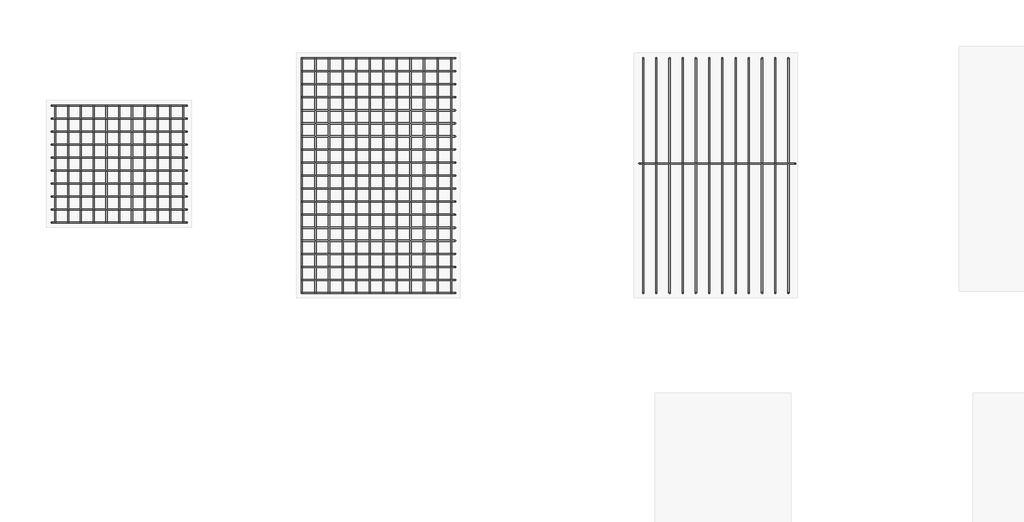
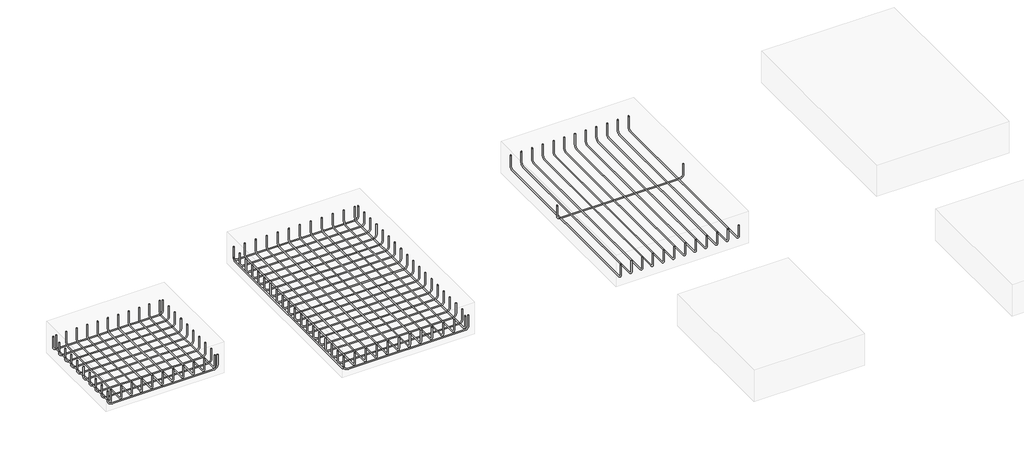
# One storey, part 2 of 2: 6 reinforcing bars.
"""IFC4 building model written with IfcOpenShell, lengths in millimetres."""

from ifc_helpers import new_model, si_unit, point, frame, origin, place, context, project, spatial, polyline, circle_curve, trimmed, segment, composite_curve, source, transform, mapped, element, save
from ifc_brep_helpers import swept_disk

model = new_model("IFC4")

# Units and contexts
model_context = context("Model", 3, world=origin())
ifc_project = project(units=[si_unit("LENGTHUNIT", "METRE", prefix="MILLI")], contexts=[model_context])

# Site, building, storey
site = spatial("IfcSite", under=ifc_project)
building = spatial("IfcBuilding", under=site)
storey = spatial("IfcBuildingStorey", under=building, Elevation=-2133.6)

# Reinforcing bars
placement = place(None, origin())
reinforcing_bar_shape = source(origin(), model_context, "Body", "SolidModel", [
    swept_disk(composite_curve([segment(polyline([(-14776.9377753, 5351.4047256, -2333.6), (-14776.9377753, 5351.4047256, -2480.9)]), True, "CONTINUOUS"), segment(trimmed(circle_curve(frame((-14823.2877753, 5351.4047256, -2480.9), z_axis=(0.0, 1.0, 0.0), x_axis=(46.349999999998545, 0.0, 0.0)), 46.35), [point((-14776.9377753, 5351.4047256, -2480.9))], [point((-14823.2877753, 5351.4047256, -2527.25))], True, "CARTESIAN"), True, "CONTINUOUS"), segment(polyline([(-14823.2877753, 5351.4047256, -2527.25), (-16217.8877753, 5351.4047256, -2527.25)]), True, "CONTINUOUS"), segment(trimmed(circle_curve(frame((-16217.8877753, 5351.4047256, -2480.9), z_axis=(0.0, 1.0, 0.0), x_axis=(0.0, 0.0, -46.34999999999991)), 46.35), [point((-16217.8877753, 5351.4047256, -2527.25))], [point((-16264.2377753, 5351.4047256, -2480.9))], True, "CARTESIAN"), True, "CONTINUOUS"), segment(polyline([(-16264.2377753, 5351.4047256, -2480.9), (-16264.2377753, 5351.4047256, -2333.6)]), True, "CONTINUOUS")], self_intersect=False), 6.35),
])
element("IfcReinforcingBar", 1, at=placement, inside=storey, context=model_context, shape_type="MappedRepresentation", body=[
    mapped(reinforcing_bar_shape, transform((0.0, 0.0, 0.0), x_axis=(1.0, 0.0, 0.0), y_axis=(0.0, 1.0, 0.0), z_axis=(0.0, 0.0, 1.0))),
    mapped(reinforcing_bar_shape, transform((0.0, -143.0333333, 0.0), x_axis=(1.0, 0.0, 0.0), y_axis=(0.0, 1.0, 0.0), z_axis=(0.0, 0.0, 1.0))),
    mapped(reinforcing_bar_shape, transform((0.0, -286.0666667, 0.0), x_axis=(1.0, 0.0, 0.0), y_axis=(0.0, 1.0, 0.0), z_axis=(0.0, 0.0, 1.0))),
    mapped(reinforcing_bar_shape, transform((0.0, -429.1, 0.0), x_axis=(1.0, 0.0, 0.0), y_axis=(0.0, 1.0, 0.0), z_axis=(0.0, 0.0, 1.0))),
    mapped(reinforcing_bar_shape, transform((0.0, -572.1333333, 0.0), x_axis=(1.0, 0.0, 0.0), y_axis=(0.0, 1.0, 0.0), z_axis=(0.0, 0.0, 1.0))),
    mapped(reinforcing_bar_shape, transform((0.0, -715.1666667, 0.0), x_axis=(1.0, 0.0, 0.0), y_axis=(0.0, 1.0, 0.0), z_axis=(0.0, 0.0, 1.0))),
    mapped(reinforcing_bar_shape, transform((0.0, -858.2, 0.0), x_axis=(1.0, 0.0, 0.0), y_axis=(0.0, 1.0, 0.0), z_axis=(0.0, 0.0, 1.0))),
    mapped(reinforcing_bar_shape, transform((0.0, -1001.2333333, 0.0), x_axis=(1.0, 0.0, 0.0), y_axis=(0.0, 1.0, 0.0), z_axis=(0.0, 0.0, 1.0))),
    mapped(reinforcing_bar_shape, transform((0.0, -1144.2666667, 0.0), x_axis=(1.0, 0.0, 0.0), y_axis=(0.0, 1.0, 0.0), z_axis=(0.0, 0.0, 1.0))),
    mapped(reinforcing_bar_shape, transform((0.0, -1287.3, 0.0), x_axis=(1.0, 0.0, 0.0), y_axis=(0.0, 1.0, 0.0), z_axis=(0.0, 0.0, 1.0))),
])
reinforcing_bar_2_shape = source(origin(), model_context, "Body", "SolidModel", [
    swept_disk(composite_curve([segment(polyline([(-16224.2377753, 5351.4047256, -2327.3038613), (-16224.2377753, 5351.4047256, -2474.6038613)]), True, "CONTINUOUS"), segment(trimmed(circle_curve(frame((-16224.2377753, 5305.0547256, -2474.6038613), z_axis=(-1.0, 0.0, 0.0), x_axis=(0.0, 46.350000000000364, 0.0)), 46.35), [point((-16224.2377753, 5351.4047256, -2474.6038613))], [point((-16224.2377753, 5305.0547256, -2520.9538613))], True, "CARTESIAN"), True, "CONTINUOUS"), segment(polyline([(-16224.2377753, 5305.0547256, -2520.9538613), (-16224.2377753, 4110.4547256, -2520.9538613)]), True, "CONTINUOUS"), segment(trimmed(circle_curve(frame((-16224.2377753, 4110.4547256, -2474.6038613), z_axis=(-1.0, 0.0, 0.0), x_axis=(0.0, 0.0, -46.34999999999991)), 46.35), [point((-16224.2377753, 4110.4547256, -2520.9538613))], [point((-16224.2377753, 4064.1047256, -2474.6038613))], True, "CARTESIAN"), True, "CONTINUOUS"), segment(polyline([(-16224.2377753, 4064.1047256, -2474.6038613), (-16224.2377753, 4064.1047256, -2327.3038613)]), True, "CONTINUOUS")], self_intersect=False), 6.35),
])
element("IfcReinforcingBar", 2, at=placement, inside=storey, context=model_context, shape_type="MappedRepresentation", body=[
    mapped(reinforcing_bar_2_shape, transform((0.0, 0.0, 0.0), x_axis=(1.0, 0.0, 0.0), y_axis=(0.0, 1.0, 0.0), z_axis=(0.0, 0.0, 1.0))),
    mapped(reinforcing_bar_2_shape, transform((140.73, 0.0, 0.0), x_axis=(1.0, 0.0, 0.0), y_axis=(0.0, 1.0, 0.0), z_axis=(0.0, 0.0, 1.0))),
    mapped(reinforcing_bar_2_shape, transform((281.46, 0.0, 0.0), x_axis=(1.0, 0.0, 0.0), y_axis=(0.0, 1.0, 0.0), z_axis=(0.0, 0.0, 1.0))),
    mapped(reinforcing_bar_2_shape, transform((422.19, 0.0, 0.0), x_axis=(1.0, 0.0, 0.0), y_axis=(0.0, 1.0, 0.0), z_axis=(0.0, 0.0, 1.0))),
    mapped(reinforcing_bar_2_shape, transform((562.92, 0.0, 0.0), x_axis=(1.0, 0.0, 0.0), y_axis=(0.0, 1.0, 0.0), z_axis=(0.0, 0.0, 1.0))),
    mapped(reinforcing_bar_2_shape, transform((703.65, 0.0, 0.0), x_axis=(1.0, 0.0, 0.0), y_axis=(0.0, 1.0, 0.0), z_axis=(0.0, 0.0, 1.0))),
    mapped(reinforcing_bar_2_shape, transform((844.38, 0.0, 0.0), x_axis=(1.0, 0.0, 0.0), y_axis=(0.0, 1.0, 0.0), z_axis=(0.0, 0.0, 1.0))),
    mapped(reinforcing_bar_2_shape, transform((985.11, 0.0, 0.0), x_axis=(1.0, 0.0, 0.0), y_axis=(0.0, 1.0, 0.0), z_axis=(0.0, 0.0, 1.0))),
    mapped(reinforcing_bar_2_shape, transform((1125.84, 0.0, 0.0), x_axis=(1.0, 0.0, 0.0), y_axis=(0.0, 1.0, 0.0), z_axis=(0.0, 0.0, 1.0))),
    mapped(reinforcing_bar_2_shape, transform((1266.57, 0.0, 0.0), x_axis=(1.0, 0.0, 0.0), y_axis=(0.0, 1.0, 0.0), z_axis=(0.0, 0.0, 1.0))),
    mapped(reinforcing_bar_2_shape, transform((1407.3, 0.0, 0.0), x_axis=(1.0, 0.0, 0.0), y_axis=(0.0, 1.0, 0.0), z_axis=(0.0, 0.0, 1.0))),
])
reinforcing_bar_3_shape = source(origin(), model_context, "Body", "SolidModel", [
    swept_disk(composite_curve([segment(polyline([(-11823.152732, 5876.4047256, -2333.6), (-11823.152732, 5876.4047256, -2480.9)]), True, "CONTINUOUS"), segment(trimmed(circle_curve(frame((-11869.502732, 5876.4047256, -2480.9), z_axis=(0.0, 1.0, 0.0), x_axis=(46.350000000000364, 0.0, 0.0)), 46.35), [point((-11823.152732, 5876.4047256, -2480.9))], [point((-11869.502732, 5876.4047256, -2527.25))], True, "CARTESIAN"), True, "CONTINUOUS"), segment(polyline([(-11869.502732, 5876.4047256, -2527.25), (-13464.102732, 5876.4047256, -2527.25)]), True, "CONTINUOUS"), segment(trimmed(circle_curve(frame((-13464.102732, 5876.4047256, -2480.9), z_axis=(0.0, 1.0, 0.0), x_axis=(0.0, 0.0, -46.34999999999991)), 46.35), [point((-13464.102732, 5876.4047256, -2527.25))], [point((-13510.452732, 5876.4047256, -2480.9))], True, "CARTESIAN"), True, "CONTINUOUS"), segment(polyline([(-13510.452732, 5876.4047256, -2480.9), (-13510.452732, 5876.4047256, -2333.6)]), True, "CONTINUOUS")], self_intersect=False), 6.35),
])
element("IfcReinforcingBar", 3, at=placement, inside=storey, context=model_context, shape_type="MappedRepresentation", body=[
    mapped(reinforcing_bar_3_shape, transform((0.0, 0.0, 0.0), x_axis=(1.0, 0.0, 0.0), y_axis=(0.0, 1.0, 0.0), z_axis=(0.0, 0.0, 1.0))),
    mapped(reinforcing_bar_3_shape, transform((0.0, -143.7388889, 0.0), x_axis=(1.0, 0.0, 0.0), y_axis=(0.0, 1.0, 0.0), z_axis=(0.0, 0.0, 1.0))),
    mapped(reinforcing_bar_3_shape, transform((0.0, -287.4777778, 0.0), x_axis=(1.0, 0.0, 0.0), y_axis=(0.0, 1.0, 0.0), z_axis=(0.0, 0.0, 1.0))),
    mapped(reinforcing_bar_3_shape, transform((0.0, -431.2166667, 0.0), x_axis=(1.0, 0.0, 0.0), y_axis=(0.0, 1.0, 0.0), z_axis=(0.0, 0.0, 1.0))),
    mapped(reinforcing_bar_3_shape, transform((0.0, -574.9555556, 0.0), x_axis=(1.0, 0.0, 0.0), y_axis=(0.0, 1.0, 0.0), z_axis=(0.0, 0.0, 1.0))),
    mapped(reinforcing_bar_3_shape, transform((0.0, -718.6944444, 0.0), x_axis=(1.0, 0.0, 0.0), y_axis=(0.0, 1.0, 0.0), z_axis=(0.0, 0.0, 1.0))),
    mapped(reinforcing_bar_3_shape, transform((0.0, -862.4333333, 0.0), x_axis=(1.0, 0.0, 0.0), y_axis=(0.0, 1.0, 0.0), z_axis=(0.0, 0.0, 1.0))),
    mapped(reinforcing_bar_3_shape, transform((0.0, -1006.1722222, 0.0), x_axis=(1.0, 0.0, 0.0), y_axis=(0.0, 1.0, 0.0), z_axis=(0.0, 0.0, 1.0))),
    mapped(reinforcing_bar_3_shape, transform((0.0, -1149.9111111, 0.0), x_axis=(1.0, 0.0, 0.0), y_axis=(0.0, 1.0, 0.0), z_axis=(0.0, 0.0, 1.0))),
    mapped(reinforcing_bar_3_shape, transform((0.0, -1293.65, 0.0), x_axis=(1.0, 0.0, 0.0), y_axis=(0.0, 1.0, 0.0), z_axis=(0.0, 0.0, 1.0))),
    mapped(reinforcing_bar_3_shape, transform((0.0, -1437.3888889, 0.0), x_axis=(1.0, 0.0, 0.0), y_axis=(0.0, 1.0, 0.0), z_axis=(0.0, 0.0, 1.0))),
    mapped(reinforcing_bar_3_shape, transform((0.0, -1581.1277778, 0.0), x_axis=(1.0, 0.0, 0.0), y_axis=(0.0, 1.0, 0.0), z_axis=(0.0, 0.0, 1.0))),
    mapped(reinforcing_bar_3_shape, transform((0.0, -1724.8666667, 0.0), x_axis=(1.0, 0.0, 0.0), y_axis=(0.0, 1.0, 0.0), z_axis=(0.0, 0.0, 1.0))),
    mapped(reinforcing_bar_3_shape, transform((0.0, -1868.6055556, 0.0), x_axis=(1.0, 0.0, 0.0), y_axis=(0.0, 1.0, 0.0), z_axis=(0.0, 0.0, 1.0))),
    mapped(reinforcing_bar_3_shape, transform((0.0, -2012.3444444, 0.0), x_axis=(1.0, 0.0, 0.0), y_axis=(0.0, 1.0, 0.0), z_axis=(0.0, 0.0, 1.0))),
    mapped(reinforcing_bar_3_shape, transform((0.0, -2156.0833333, 0.0), x_axis=(1.0, 0.0, 0.0), y_axis=(0.0, 1.0, 0.0), z_axis=(0.0, 0.0, 1.0))),
    mapped(reinforcing_bar_3_shape, transform((0.0, -2299.8222222, 0.0), x_axis=(1.0, 0.0, 0.0), y_axis=(0.0, 1.0, 0.0), z_axis=(0.0, 0.0, 1.0))),
    mapped(reinforcing_bar_3_shape, transform((0.0, -2443.5611111, 0.0), x_axis=(1.0, 0.0, 0.0), y_axis=(0.0, 1.0, 0.0), z_axis=(0.0, 0.0, 1.0))),
    mapped(reinforcing_bar_3_shape, transform((0.0, -2587.3, 0.0), x_axis=(1.0, 0.0, 0.0), y_axis=(0.0, 1.0, 0.0), z_axis=(0.0, 0.0, 1.0))),
])
reinforcing_bar_4_shape = source(origin(), model_context, "Body", "SolidModel", [
    swept_disk(composite_curve([segment(polyline([(-13510.452732, 5876.4047256, -2327.2198924), (-13510.452732, 5876.4047256, -2474.5198924)]), True, "CONTINUOUS"), segment(trimmed(circle_curve(frame((-13510.452732, 5830.0547256, -2474.5198924), z_axis=(-1.0, 0.0, 0.0), x_axis=(0.0, 46.350000000000364, 0.0)), 46.35), [point((-13510.452732, 5876.4047256, -2474.5198924))], [point((-13510.452732, 5830.0547256, -2520.8698924))], True, "CARTESIAN"), True, "CONTINUOUS"), segment(polyline([(-13510.452732, 5830.0547256, -2520.8698924), (-13510.452732, 3335.4547256, -2520.8698924)]), True, "CONTINUOUS"), segment(trimmed(circle_curve(frame((-13510.452732, 3335.4547256, -2474.5198924), z_axis=(-1.0, 0.0, 0.0), x_axis=(0.0, 0.0, -46.34999999999991)), 46.35), [point((-13510.452732, 3335.4547256, -2520.8698924))], [point((-13510.452732, 3289.1047256, -2474.5198924))], True, "CARTESIAN"), True, "CONTINUOUS"), segment(polyline([(-13510.452732, 3289.1047256, -2474.5198924), (-13510.452732, 3289.1047256, -2327.2198924)]), True, "CONTINUOUS")], self_intersect=False), 6.35),
])
element("IfcReinforcingBar", 4, at=placement, inside=storey, context=model_context, shape_type="MappedRepresentation", body=[
    mapped(reinforcing_bar_4_shape, transform((0.0, 0.0, 0.0), x_axis=(1.0, 0.0, 0.0), y_axis=(0.0, 1.0, 0.0), z_axis=(0.0, 0.0, 1.0))),
    mapped(reinforcing_bar_4_shape, transform((149.4666138, 0.0, 0.0), x_axis=(1.0, 0.0, 0.0), y_axis=(0.0, 1.0, 0.0), z_axis=(0.0, 0.0, 1.0))),
    mapped(reinforcing_bar_4_shape, transform((298.9332277, 0.0, 0.0), x_axis=(1.0, 0.0, 0.0), y_axis=(0.0, 1.0, 0.0), z_axis=(0.0, 0.0, 1.0))),
    mapped(reinforcing_bar_4_shape, transform((448.3998415, 0.0, 0.0), x_axis=(1.0, 0.0, 0.0), y_axis=(0.0, 1.0, 0.0), z_axis=(0.0, 0.0, 1.0))),
    mapped(reinforcing_bar_4_shape, transform((597.8664554, 0.0, 0.0), x_axis=(1.0, 0.0, 0.0), y_axis=(0.0, 1.0, 0.0), z_axis=(0.0, 0.0, 1.0))),
    mapped(reinforcing_bar_4_shape, transform((747.3330692, 0.0, 0.0), x_axis=(1.0, 0.0, 0.0), y_axis=(0.0, 1.0, 0.0), z_axis=(0.0, 0.0, 1.0))),
    mapped(reinforcing_bar_4_shape, transform((896.7996831, 0.0, 0.0), x_axis=(1.0, 0.0, 0.0), y_axis=(0.0, 1.0, 0.0), z_axis=(0.0, 0.0, 1.0))),
    mapped(reinforcing_bar_4_shape, transform((1046.2662969, 0.0, 0.0), x_axis=(1.0, 0.0, 0.0), y_axis=(0.0, 1.0, 0.0), z_axis=(0.0, 0.0, 1.0))),
    mapped(reinforcing_bar_4_shape, transform((1195.7329107, 0.0, 0.0), x_axis=(1.0, 0.0, 0.0), y_axis=(0.0, 1.0, 0.0), z_axis=(0.0, 0.0, 1.0))),
    mapped(reinforcing_bar_4_shape, transform((1345.1995246, 0.0, 0.0), x_axis=(1.0, 0.0, 0.0), y_axis=(0.0, 1.0, 0.0), z_axis=(0.0, 0.0, 1.0))),
    mapped(reinforcing_bar_4_shape, transform((1494.6661384, 0.0, 0.0), x_axis=(1.0, 0.0, 0.0), y_axis=(0.0, 1.0, 0.0), z_axis=(0.0, 0.0, 1.0))),
    mapped(reinforcing_bar_4_shape, transform((1644.1327523, 0.0, 0.0), x_axis=(1.0, 0.0, 0.0), y_axis=(0.0, 1.0, 0.0), z_axis=(0.0, 0.0, 1.0))),
])
element("IfcReinforcingBar", 5, at=placement, inside=storey, context=model_context, shape_type="SolidModel", body=[
    swept_disk(composite_curve([segment(polyline([(-8080.4943343, 4715.9290541, -2333.6), (-8080.4943343, 4715.9290541, -2480.9)]), True, "CONTINUOUS"), segment(trimmed(circle_curve(frame((-8126.8443343, 4715.9290541, -2480.9), z_axis=(0.0, 1.0, 0.0), x_axis=(46.349999999999454, 0.0, 0.0)), 46.35), [point((-8080.4943343, 4715.9290541, -2480.9))], [point((-8126.8443343, 4715.9290541, -2527.25))], True, "CARTESIAN"), True, "CONTINUOUS"), segment(polyline([(-8126.8443343, 4715.9290541, -2527.25), (-9747.602732, 4715.9290541, -2527.25)]), True, "CONTINUOUS"), segment(trimmed(circle_curve(frame((-9747.602732, 4715.9290541, -2480.9), z_axis=(0.0, 1.0, 0.0), x_axis=(0.0, 0.0, -46.34999999999991)), 46.35), [point((-9747.602732, 4715.9290541, -2527.25))], [point((-9793.952732, 4715.9290541, -2480.9))], True, "CARTESIAN"), True, "CONTINUOUS"), segment(polyline([(-9793.952732, 4715.9290541, -2480.9), (-9793.952732, 4715.9290541, -2333.6)]), True, "CONTINUOUS")], self_intersect=False), 6.35),
])
reinforcing_bar_5_shape = source(origin(), model_context, "Body", "SolidModel", [
    swept_disk(composite_curve([segment(polyline([(-9753.952732, 5876.4047256, -2327.2775664), (-9753.952732, 5876.4047256, -2474.5775664)]), True, "CONTINUOUS"), segment(trimmed(circle_curve(frame((-9753.952732, 5830.0547256, -2474.5775664), z_axis=(-1.0, 0.0, 0.0), x_axis=(0.0, 46.350000000000364, 0.0)), 46.35), [point((-9753.952732, 5876.4047256, -2474.5775664))], [point((-9753.952732, 5830.0547256, -2520.9275664))], True, "CARTESIAN"), True, "CONTINUOUS"), segment(polyline([(-9753.952732, 5830.0547256, -2520.9275664), (-9753.952732, 3335.4547256, -2520.9275664)]), True, "CONTINUOUS"), segment(trimmed(circle_curve(frame((-9753.952732, 3335.4547256, -2474.5775664), z_axis=(-1.0, 0.0, 0.0), x_axis=(0.0, 0.0, -46.350000000000364)), 46.35), [point((-9753.952732, 3335.4547256, -2520.9275664))], [point((-9753.952732, 3289.1047256, -2474.5775664))], True, "CARTESIAN"), True, "CONTINUOUS"), segment(polyline([(-9753.952732, 3289.1047256, -2474.5775664), (-9753.952732, 3289.1047256, -2327.2775664)]), True, "CONTINUOUS")], self_intersect=False), 6.35),
])
element("IfcReinforcingBar", 6, at=placement, inside=storey, context=model_context, shape_type="MappedRepresentation", body=[
    mapped(reinforcing_bar_5_shape, transform((0.0, 0.0, 0.0), x_axis=(1.0, 0.0, 0.0), y_axis=(0.0, 1.0, 0.0), z_axis=(0.0, 0.0, 1.0))),
    mapped(reinforcing_bar_5_shape, transform((145.4020607, 0.0, 0.0), x_axis=(1.0, 0.0, 0.0), y_axis=(0.0, 1.0, 0.0), z_axis=(0.0, 0.0, 1.0))),
    mapped(reinforcing_bar_5_shape, transform((290.8041214, 0.0, 0.0), x_axis=(1.0, 0.0, 0.0), y_axis=(0.0, 1.0, 0.0), z_axis=(0.0, 0.0, 1.0))),
    mapped(reinforcing_bar_5_shape, transform((436.2061821, 0.0, 0.0), x_axis=(1.0, 0.0, 0.0), y_axis=(0.0, 1.0, 0.0), z_axis=(0.0, 0.0, 1.0))),
    mapped(reinforcing_bar_5_shape, transform((581.6082427, 0.0, 0.0), x_axis=(1.0, 0.0, 0.0), y_axis=(0.0, 1.0, 0.0), z_axis=(0.0, 0.0, 1.0))),
    mapped(reinforcing_bar_5_shape, transform((727.0103034, 0.0, 0.0), x_axis=(1.0, 0.0, 0.0), y_axis=(0.0, 1.0, 0.0), z_axis=(0.0, 0.0, 1.0))),
    mapped(reinforcing_bar_5_shape, transform((872.4123641, 0.0, 0.0), x_axis=(1.0, 0.0, 0.0), y_axis=(0.0, 1.0, 0.0), z_axis=(0.0, 0.0, 1.0))),
    mapped(reinforcing_bar_5_shape, transform((1017.8144248, 0.0, 0.0), x_axis=(1.0, 0.0, 0.0), y_axis=(0.0, 1.0, 0.0), z_axis=(0.0, 0.0, 1.0))),
    mapped(reinforcing_bar_5_shape, transform((1163.2164855, 0.0, 0.0), x_axis=(1.0, 0.0, 0.0), y_axis=(0.0, 1.0, 0.0), z_axis=(0.0, 0.0, 1.0))),
    mapped(reinforcing_bar_5_shape, transform((1308.6185462, 0.0, 0.0), x_axis=(1.0, 0.0, 0.0), y_axis=(0.0, 1.0, 0.0), z_axis=(0.0, 0.0, 1.0))),
    mapped(reinforcing_bar_5_shape, transform((1454.0206069, 0.0, 0.0), x_axis=(1.0, 0.0, 0.0), y_axis=(0.0, 1.0, 0.0), z_axis=(0.0, 0.0, 1.0))),
    mapped(reinforcing_bar_5_shape, transform((1599.4226676, 0.0, 0.0), x_axis=(1.0, 0.0, 0.0), y_axis=(0.0, 1.0, 0.0), z_axis=(0.0, 0.0, 1.0))),
])

save(model, "model.ifc")

# Revit data of these elements
# Elements 1, 2, 3, 4, 5, 6 (IfcReinforcingBar)
#   Phase Created = New Construction
